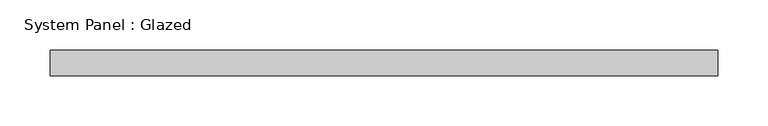
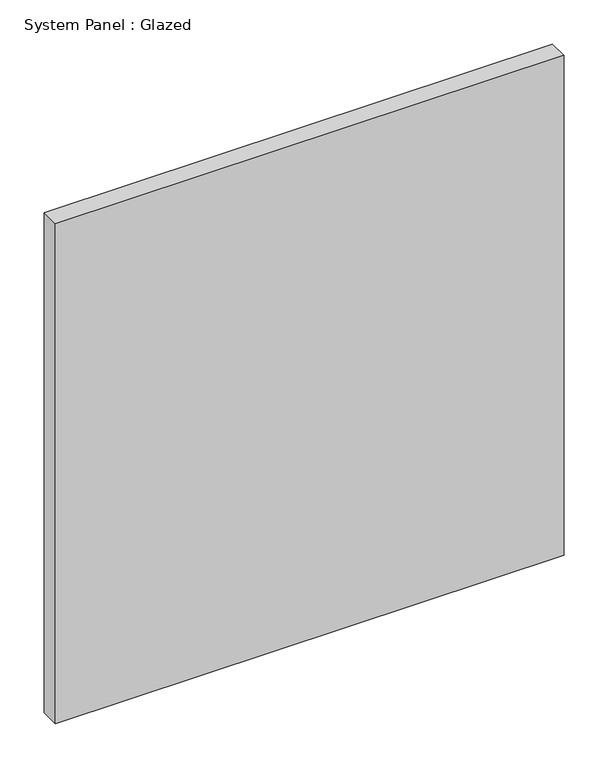
"""IFC4 building model written with IfcOpenShell, lengths in millimetres: plate geometry, System Panel : Glazed."""

from ifc_helpers import new_model, si_unit, origin, origin_with_axes, place, context, project, spatial, polyline, outline, extrude, source, transform, mapped, element, save


def system_panel_glazed_52d1a9ac(model_context):
    return source(origin(), model_context, "Body", "SweptSolid", [
        extrude(outline(polyline([(333.375, 19.05), (-333.375, 19.05), (-333.375, 44.45), (333.375, 44.45), (333.375, 19.05)])), origin_with_axes(), (0.0, 0.0, 1.0), 692.8489237),
    ])


if __name__ == "__main__":
    model = new_model("IFC4")
    model_context = context("Model", 3, world=origin())
    ifc_project = project(units=[si_unit("LENGTHUNIT", "METRE", prefix="MILLI")], contexts=[model_context])
    site = spatial("IfcSite", under=ifc_project)
    building = spatial("IfcBuilding", under=site)
    placement = place(None, origin())
    system_panel_glazed_shape = system_panel_glazed_52d1a9ac(model_context)
    element("IfcPlate", 1, ObjectType="System Panel : Glazed", at=placement, inside=building, context=model_context, shape_type="MappedRepresentation", body=[
        mapped(system_panel_glazed_shape, transform((0.0, 0.0, 0.0), x_axis=(1.0, 0.0, 0.0), y_axis=(0.0, 1.0, 0.0), z_axis=(0.0, 0.0, 1.0))),
    ])
    save(model, "model.ifc")

# Revit data of these elements
# Type "System Panel : Glazed"
#   Construction Type Id = "GSP4R"
#   Analytic Construction = "1/8 in Pilkington single glazing"
#   Visual Light Transmittance = 0.9
#   Solar Heat Gain Coefficient = 0.86
#   Heat Transfer Coefficient (U) = 1.18115 BTU/(h·ft²·°F)
#   Define Thermal Properties by = 1
# Element 1 (IfcPlate, "System Panel : Glazed")
#   Materials on its faces: "Glass"
# Materials
#   "Glass": class "Glass", colour RGB 0 128 192, transparency 0.75, Description = "Soda Lime Glass", Cost = 0
